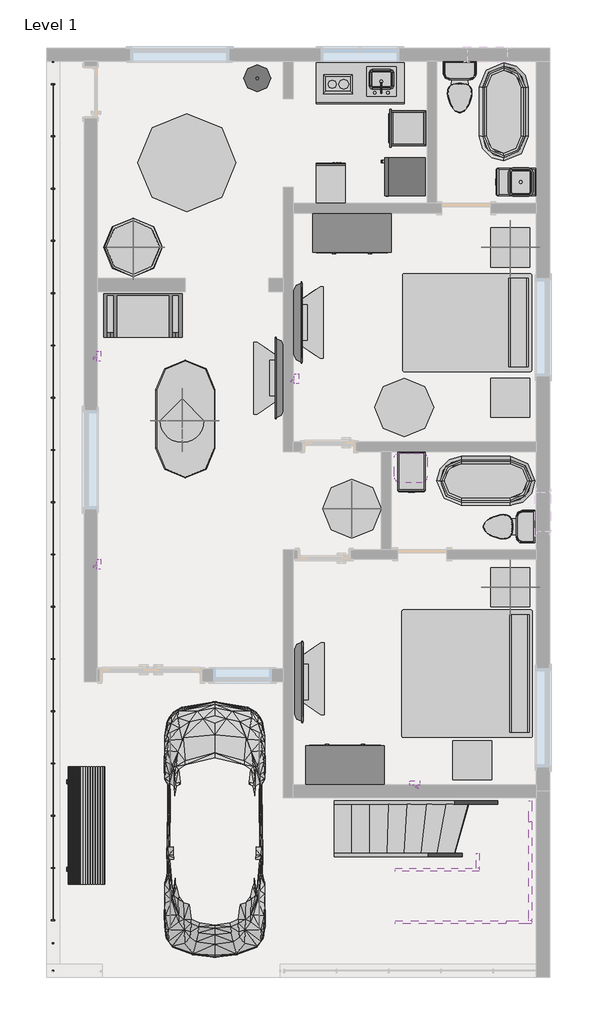
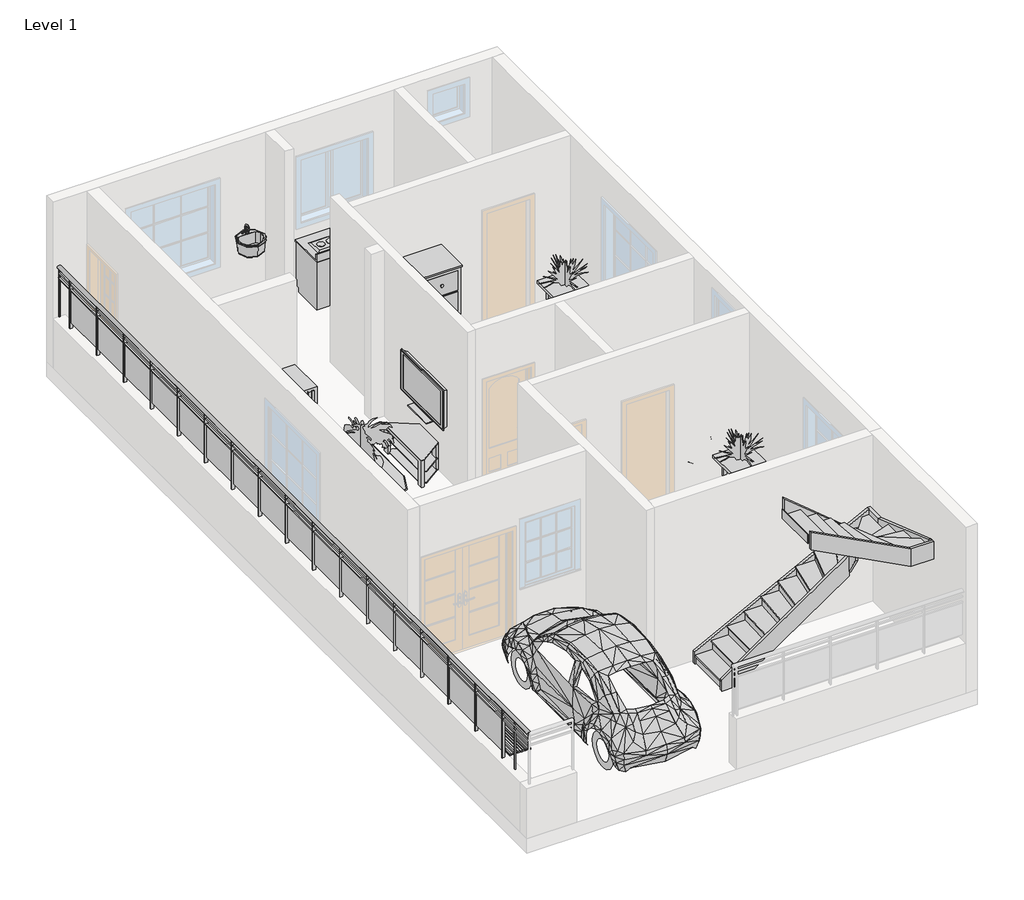
# One storey, part 2 of 2: 23 furniture elements, 10 proxies, 8 flow terminals, 8 members, 6 geographic elements, 1 railing, 1 stair flight.
# Revit data of these elements (continued)
# Elements 19, 20 (IfcFurniture, "24\"") (continued)
#   Materials on its faces: "Cabinets", "Cabinets - Handles"
# Element 21 (IfcFurniture, "Bed-Standard.0001 : King 78\" x 80\"")
#   Phase Created = New Construction
#   Materials on its faces: "Linen, White", "Steel, Chrome Plated"
# Element 22 (IfcFurniture, "Bed-Standard.0001 : Queen 60\" x 79\"")
#   Phase Created = New Construction
#   Materials on its faces: "Linen, White", "Steel, Chrome Plated"
# Element 23 (IfcFurniture, "Counter Top w Sink Hole : 24\" Depth")
#   Sink Opening Depth = 1' - 3"
#   Sink Location To Wall = 0' - 6"
#   Length = 4' - 6"
#   Sink Location = 1' - 2"
#   Sink Opening Width = 1' - 4"
#   Phase Created = New Construction
#   Materials on its faces: "Counter Top"
# Elements 24, 25 (IfcFurniture, "Dresser : 48\" x 72\" x 24\"")
#   Phase Created = New Construction
#   Materials on its faces: "Laminate, Ivory, Matte", "Cherry", "Laminate - Ivory, Glossy"
# Element 26 (IfcFurniture, "Entertainment Center : 72\" x 72\" x 24\"")
#   Phase Created = New Construction
#   Materials on its faces: "Steel, Chrome Plated", "Glass - Clear, Grey"
# Elements 27, 28, 29 (IfcFurniture, "TV - Flat Screen : 50\"")
#   Stand = yes
#   Phase Created = New Construction
#   Materials on its faces: "TV - Black", "TV - Glass", "TV - Screen"
# Elements 30, 31, 32 (IfcFurniture, "TV Stand : TV Stand")
#   Phase Created = New Construction
#   Materials on its faces: "Melamine - Gray", "Glass - Shelves"
# Element 33 (IfcFurniture, "Table-Dining Oval : 36\" x 72\"")
#   Phase Created = New Construction
#   Materials on its faces: "Steel, Chrome Plated", "Glass - Clear, Grey"
# Element 34 (IfcFurniture, "Table-Dining Round w Chairs : 60\" Diameter")
#   Phase Created = New Construction
#   Materials on its faces: "Pine", "Laminate, Linen, Matte"
# Element 35 (IfcFurniture, "Table-Ellipse : 60\" x 48\"")
#   Phase Created = New Construction
#   Materials on its faces: "Birch"
# Element 36 (IfcFurniture, "Table-Ellipse : 72\" x 36\"")
#   Phase Created = New Construction
#   Materials on its faces: "Birch", "Laminate - Black"
# Elements 37, 38, 39, 40 (IfcFurniture, "Table-Night Stand : 24\" x 24\" x 30\"")
#   Phase Created = New Construction
#   Materials on its faces: "Birch", "Laminate, Ivory, Matte"
# Element 41 (IfcFurniture, "Table-Round : 36\" Diameter")
#   Phase Created = New Construction
#   Materials on its faces: "Steel, Chrome Plated", "Birch"
# Element 42 (IfcGeographicElement, "Park Bench : 72\"")
#   Phase Created = New Construction
#   Materials on its faces: "Wood - Teak", "Steel, Paint Finish, Dark Gray, Matte"
# Element 43 (IfcGeographicElement, "RPC Plant - Tropical")
#   Phase Created = New Construction
# Elements 44, 45, 46 (IfcGeographicElement, "RPC Plant - Tropical : Agave - 1.5'")
#   Phase Created = New Construction
# Element 47 (IfcGeographicElement, "RPC Plant - Tropical : Japanese Fern - 2.5'")
#   Phase Created = New Construction
# Elements 48, 49, 50, 51, 52, 53, 54, 55 (IfcMember, "Stringer - 2\" Width")
#   Phase Created = New Construction
# Element 56 (IfcRailing, "Glass Panel - Bottom Fill")
#   built-in parameter 1008621 = 3 (stored number, unit not read)
#   Phase Created = New Construction
#   Materials on its faces: "Glass"
# Element 57 (IfcStairFlight, "2\" Tread 1\" Nosing 1/4\" Riser")
#   Phase Created = New Construction
# Materials
#   "Plastic, Opaque Black": class "Plastic", colour RGB 0 0 0, transparency 0.7, Description = "Plastic, generic, opaque black", Cost = 0
#   "Steel, Paint Finish, Ivory, Matte": class "Metal", colour RGB 247 247 239, transparency 0, Description = "Steel, paint finish, ivory, matte", Cost = 0
#   "Steel, Chrome Plated": class "Metal", colour RGB 17 17 17, transparency 0, Description = "Chromiuim plated steel", Cost = 0
#   "Steel, Polished": class "Metal", colour RGB 57 57 57, transparency 0, Description = "Polished steel", Cost = 0
#   "Cabinets": colour RGB 249 249 249, transparency 0
#   "Cabinets - Handles": class "Metal", colour RGB 57 57 57, transparency 0
#   "Metal - Stainless Steel, Polished": class "Metal", colour RGB 216 216 216, transparency 0
#   "Steel, Paint Finish, Ivory, Glossy": class "Metal", colour RGB 247 247 239, transparency 0, Description = "Steel, paint finish, ivory, glossy", Cost = 0
#   "Porcelain, Linen": class "Ceramic", colour RGB 249 239 230, transparency 0, Description = "Porcelain, linen", Cost = 0
#   "Laminate, Linen, Matte": class "Plastic", colour RGB 249 239 230, transparency 0, Description = "Plastic Laminate - Linen, Matte", Cost = 0
#   "Porcelain, Ivory": class "Ceramic", colour RGB 247 247 239, transparency 0, Description = "Porcelain, ivory", Cost = 0
#   "Linen, Beige": class "Textile", colour RGB 249 239 230, transparency 0, Description = "Linen, beige", Cost = 0
#   "Linen, White": class "Textile", colour RGB 247 247 239, transparency 0, Description = "Linen, white", Cost = 0
#   "Laminate - Ivory, Glossy": colour RGB 247 247 239, transparency 0
#   "Laminate, Ivory, Matte": class "Plastic", colour RGB 247 247 239, transparency 0, Description = "Plastic Laminate - Ivory, Matte", Cost = 0
#   "Cherry": class "Wood", colour RGB 226 177 128, transparency 0, Description = "Prunus Serotina", Cost = 0
#   "Melamine - Gray": class "Wood", colour RGB 49 49 49, transparency 0
#   "Glass - Clear, Grey": class "Glass", colour RGB 252 255 255, transparency 0.64
#   "Pine": class "Wood", colour RGB 223 192 134, transparency 0, Description = "Pinus Echinata", Cost = 0
#   "Birch": class "Wood", colour RGB 224 178 126, transparency 0, Description = "Betula Alleghaniensis", Cost = 0
#   "Laminate - Black": colour RGB 0 0 0, transparency 0
#   "Wood - Teak": class "Wood", colour RGB 120 73 19, transparency 0
#   "Steel, Paint Finish, Dark Gray, Matte": class "Metal", colour RGB 98 98 98, transparency 0, Description = "Steel, paint finish, dark gray, matte", Cost = 0
#   "Steel": class "Metal", colour RGB 247 247 247, transparency 0, Description = "Steel, mill finish", Cost = 0
#   "Glass": class "Glass", colour RGB 0 128 192, transparency 0.75, Description = "Soda Lime Glass", Cost = 0
#   "Counter Top": class "Wood", colour RGB 226 177 128, transparency 0
#   "TV - Black": colour RGB 49 49 49, transparency 0
#   "TV - Glass": colour RGB 157 157 157, transparency 0.9
#   "TV - Screen": colour RGB 0 0 0, transparency 0
#   "Glass - Shelves": class "Glass", colour RGB 167 167 167, transparency 0.9
